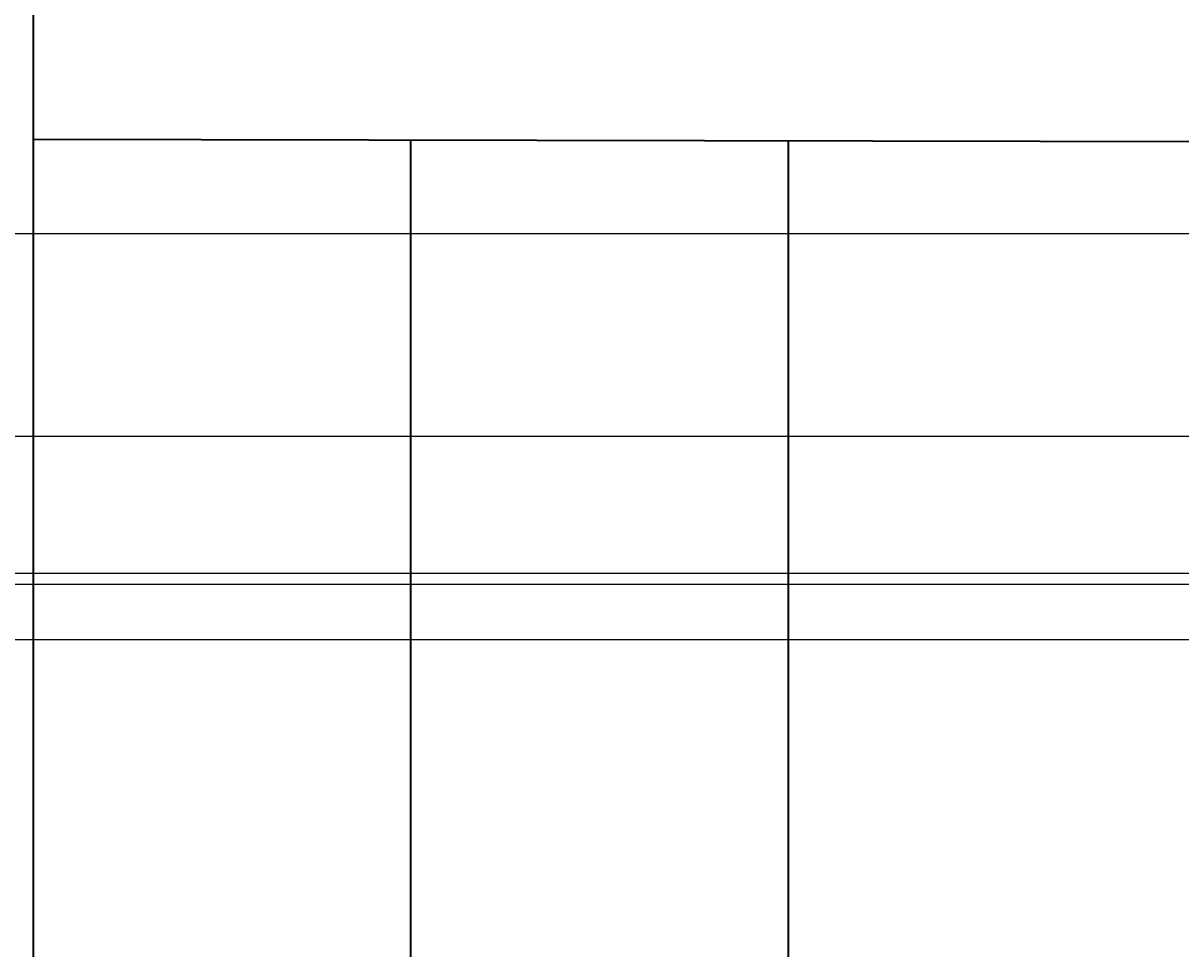
# Model space of a CAD drawing. Units: inches. Extents: x 27 to 200, y -50 to 102.
# Tile 9 of 26: x 89 to 117, y -3 to 19. Entities that reach past the tile are written whole.
import ezdxf

# ---------------------------------------------------------------- set-up
doc = ezdxf.new("R2010")
doc.units = ezdxf.units.IN
doc.header["$MEASUREMENT"] = 0
doc.layers.add('A-ANNO-DIMS', color=2, linetype='Continuous', lineweight=18)
doc.layers.add('A-ELEV', color=7, linetype='Continuous', lineweight=35)
doc.styles.get("Standard").update_dxf_attribs({"font": 'arial.ttf'})
doc.dimstyles.get("Standard").update_dxf_attribs({"dimtxt": 0.18, "dimasz": 0.18, "dimexe": 0.18, "dimexo": 0.0625, "dimgap": 0.09, "dimtad": 0, "dimtih": 1, "dimtoh": 1, "dimdec": 4, "dimzin": 0, "dimdsep": 46, "dimtxsty": 'Standard', "dimcen": 0.09, "dimadec": 0, "dimazin": 0, "dimtfac": 1, "dimtdec": 4, "dimtofl": 0, "dimtmove": 0, "dimatfit": 3, "dimfxl": 1, "dimtolj": 1, "dimtzin": 0, "dimarcsym": 0})

# ---------------------------------------------------------------- blocks, each defined once
blk = doc.blocks.new('*D48')
at = {"layer": 'A-ANNO-DIMS', "color": 0, "lineweight": -2, "transparency": 16777216}
for p, q in [((84.479, 44.926), (199.797, 44.926)), ((199.617, 44.746), (199.617, 14.26)), ((199.617, -16.589), (199.617, 13.897)), ((84.479, -16.769), (199.797, -16.769))]:
    blk.add_line(p, q, dxfattribs=at)
at = {"layer": 'A-ANNO-DIMS', "color": 0, "transparency": 16777216}
for points in [[(199.587, 44.746), (199.647, 44.746), (199.617, 44.926)], [(199.587, -16.589), (199.647, -16.589), (199.617, -16.769)]]:
    blk.add_solid(points, dxfattribs=at)
at = {"layer": 'Defpoints', "color": 0, "transparency": 16777216}
for p in [(84.417, 44.926), (199.617, 44.926), (84.417, -16.769)]:
    blk.add_point(p, dxfattribs=at)
at = {"layer": 'A-ANNO-DIMS', "color": 0, "transparency": 16777216, "insert": (199.617, 14.079), "char_height": 0.18, "attachment_point": 5}
blk.add_mtext('\\A1;61.7', dxfattribs=at)
blk = doc.blocks.new('*D54')
at = {"layer": 'A-ANNO-DIMS', "color": 0, "lineweight": -2, "transparency": 16777216}
for p, q in [((120.833, 13.977), (27.037, 13.977)), ((27.217, 13.797), (27.217, 11.743)), ((27.217, 9.324), (27.217, 11.379)), ((120.833, 9.144), (27.037, 9.144))]:
    blk.add_line(p, q, dxfattribs=at)
at = {"layer": 'A-ANNO-DIMS', "color": 0, "transparency": 16777216}
for points in [[(27.187, 13.797), (27.247, 13.797), (27.217, 13.977)], [(27.187, 9.324), (27.247, 9.324), (27.217, 9.144)]]:
    blk.add_solid(points, dxfattribs=at)
at = {"layer": 'Defpoints', "color": 0, "transparency": 16777216}
for p in [(27.217, 13.977), (120.895, 13.977), (120.895, 9.144)]:
    blk.add_point(p, dxfattribs=at)
at = {"layer": 'A-ANNO-DIMS', "color": 0, "transparency": 16777216, "insert": (27.217, 11.561), "char_height": 0.18, "attachment_point": 5}
blk.add_mtext('\\A1;4.83', dxfattribs=at)
blk = doc.blocks.new('*D56')
at = {"layer": 'A-ANNO-DIMS', "color": 0, "lineweight": -2, "transparency": 16777216}
for p, q in [((121.225, 5.878), (27.037, 5.878)), ((27.217, 5.698), (27.217, -3.085)), ((27.217, -12.231), (27.217, -3.448)), ((121.225, -12.411), (27.037, -12.411))]:
    blk.add_line(p, q, dxfattribs=at)
at = {"layer": 'A-ANNO-DIMS', "color": 0, "transparency": 16777216}
for points in [[(27.187, 5.698), (27.247, 5.698), (27.217, 5.878)], [(27.187, -12.231), (27.247, -12.231), (27.217, -12.411)]]:
    blk.add_solid(points, dxfattribs=at)
at = {"layer": 'Defpoints', "color": 0, "transparency": 16777216}
for p in [(27.217, 5.878), (121.288, 5.878), (121.288, -12.411)]:
    blk.add_point(p, dxfattribs=at)
at = {"layer": 'A-ANNO-DIMS', "color": 0, "transparency": 16777216, "insert": (27.217, -3.267), "char_height": 0.18, "attachment_point": 5}
blk.add_mtext('\\A1;18.29', dxfattribs=at)
blk = doc.blocks.new('*D68')
at = {"layer": 'A-ANNO-DIMS', "color": 0, "lineweight": -2, "transparency": 16777216}
for p, q in [((145.153, 5.617), (27.037, 5.617)), ((27.217, 5.437), (27.217, 5.138)), ((27.217, 4.476), (27.217, 4.774)), ((145.153, 4.296), (27.037, 4.296))]:
    blk.add_line(p, q, dxfattribs=at)
at = {"layer": 'A-ANNO-DIMS', "color": 0, "transparency": 16777216}
for points in [[(27.187, 5.437), (27.247, 5.437), (27.217, 5.617)], [(27.187, 4.476), (27.247, 4.476), (27.217, 4.296)]]:
    blk.add_solid(points, dxfattribs=at)
at = {"layer": 'Defpoints', "color": 0, "transparency": 16777216}
for p in [(27.217, 5.617), (145.216, 5.617), (145.216, 4.296)]:
    blk.add_point(p, dxfattribs=at)
at = {"layer": 'A-ANNO-DIMS', "color": 0, "transparency": 16777216, "insert": (27.217, 4.956), "char_height": 0.18, "attachment_point": 5}
blk.add_mtext('\\A1;1.32', dxfattribs=at)

msp = doc.modelspace()

# ---------------------------------------------------------------- linework, layer by layer
at = {"layer": 'A-ELEV'}
for p, q in [((89.3118, -16.7693), (89.3118, 19.2307)), ((191.4102, 16.002), (89.3051, 16.2307)), ((98.3118, -16.7693), (98.3118, 16.2105)), ((107.3118, -16.7693), (107.3118, 16.1904))]:
    msp.add_line(p, q, dxfattribs=at)

# ---------------------------------------------------------------- dimensions: what is measured, and where the dimension line sits
at = {"layer": 'A-ANNO-DIMS'}
for base, p1, p2, override, picture, middle in [((199.6169, 44.9264), (84.4169, -16.7693), (84.4169, 44.9264), {"dimdec": 1, "dimlfac": 1, "dimrnd": 0, "dimzin": 0, "dimdsep": 46, "dimlunit": 2}, '*D48', (199.6169, 14.0786)), ((27.2169, 13.9773), (120.8954, 9.1438), (120.8954, 13.9773), {"dimdec": 2, "dimlfac": 1, "dimrnd": 0, "dimzin": 0, "dimdsep": 46, "dimlunit": 2}, '*D54', (27.2169, 11.5606)), ((27.2169, 5.8779), (121.2876, -12.411), (121.2876, 5.8779), {"dimdec": 2, "dimlfac": 1, "dimrnd": 0, "dimzin": 0, "dimdsep": 46, "dimlunit": 2}, '*D56', (27.2169, -3.2665)), ((27.2169, 5.6167), (145.216, 4.2959), (145.216, 5.6167), {"dimdec": 2, "dimlfac": 1, "dimrnd": 0, "dimzin": 0, "dimdsep": 46, "dimlunit": 2}, '*D68', (27.2169, 4.9563))]:
    dim = msp.add_linear_dim(base=base, p1=p1, p2=p2, angle=90, dimstyle='Standard', override=override, dxfattribs=at)
    dim.commit()
    dim.dimension.update_dxf_attribs({"geometry": picture, "text_midpoint": middle})

doc.saveas('drawing.dxf')
